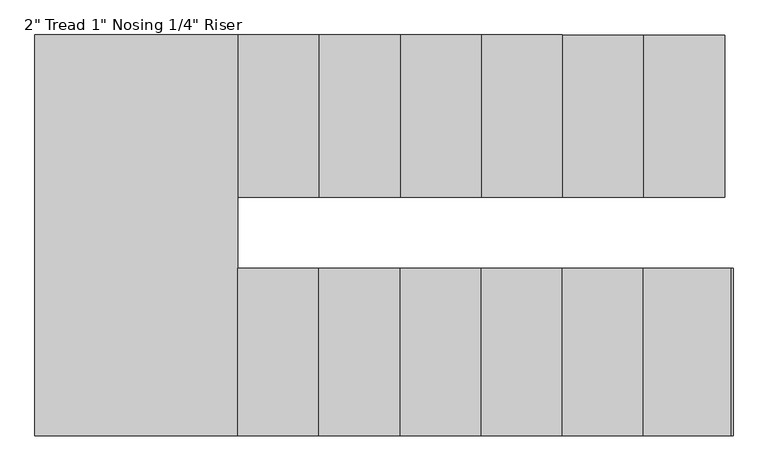
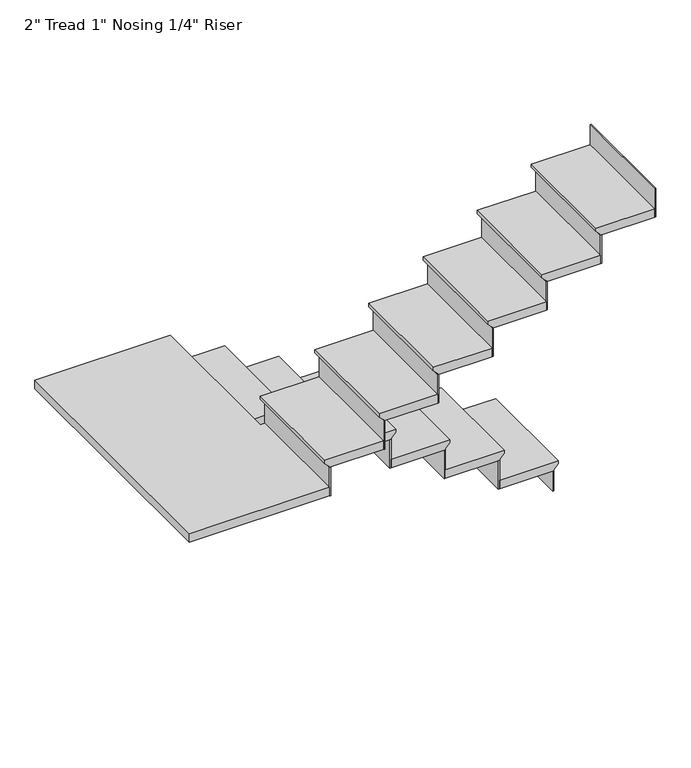
"""IFC4 building model written with IfcOpenShell, lengths in millimetres: stair flight geometry."""

from ifc_helpers import new_model, si_unit, origin, place, context, project, spatial, faceted_brep, source, transform, mapped, element, save


def stair_flight_b71cab51(model_context):
    return source(origin(), model_context, "Body", "Brep", [
        faceted_brep([(-2968.8120155, -2170.0065691, 3350.6833333), (-2968.8120155, -2170.0065691, 3369.7333333), (-2968.8120155, -2779.6065691, 3369.7333333), (-2968.8120155, -2779.6065691, 3350.6833333), (-2994.2120155, -2170.0065691, 3325.2833333), (-2994.2120155, -2779.6065691, 3325.2833333), (-3299.0120155, -2170.0065691, 3369.7333333), (-3299.0120155, -2779.6065691, 3369.7333333), (-2994.2120155, -2779.6065691, 3318.9333333), (-3299.0120155, -2779.6065691, 3318.9333333), (-3299.0120155, -2170.0065691, 3318.9333333), (-2994.2120155, -2170.0065691, 3318.9333333)], [[[0, 1, 2, 3]], [[4, 0, 3, 5]], [[2, 1, 6, 7]], [[8, 9, 10, 11]], [[2, 7, 9, 8, 5, 3]], [[8, 11, 4, 5]], [[6, 1, 0, 4, 11, 10]], [[7, 6, 10, 9]]]),
        faceted_brep([(-2994.2120155, -2170.0065691, 3318.9333333), (-2994.2120155, -2170.0065691, 3200.4), (-3000.5620155, -2170.0065691, 3200.4), (-3000.5620155, -2170.0065691, 3318.9333333), (-2994.2120155, -2779.6065691, 3318.9333333), (-3000.5620155, -2779.6065691, 3318.9333333), (-3000.5620155, -2779.6065691, 3200.4), (-2994.2120155, -2779.6065691, 3200.4)], [[[0, 1, 2, 3]], [[4, 5, 6, 7]], [[1, 0, 4, 7]], [[2, 1, 7, 6]], [[3, 2, 6, 5]], [[0, 3, 5, 4]]]),
        faceted_brep([(-3299.0120155, -2170.0065691, 3488.2666667), (-3299.0120155, -2170.0065691, 3318.9333333), (-3305.3620155, -2170.0065691, 3318.9333333), (-3305.3620155, -2170.0065691, 3488.2666667), (-3299.0120155, -2779.6065691, 3488.2666667), (-3305.3620155, -2779.6065691, 3488.2666667), (-3305.3620155, -2779.6065691, 3318.9333333), (-3299.0120155, -2779.6065691, 3318.9333333)], [[[0, 1, 2, 3]], [[4, 5, 6, 7]], [[1, 0, 4, 7]], [[2, 1, 7, 6]], [[3, 2, 6, 5]], [[0, 3, 5, 4]]]),
        faceted_brep([(-3273.6120155, -2779.6065691, 3539.0666667), (-3273.6120155, -2170.0065691, 3539.0666667), (-3603.8120155, -2170.0065691, 3539.0666667), (-3603.8120155, -2779.6065691, 3539.0666667), (-3299.0120155, -2779.6065691, 3488.2666667), (-3603.8120155, -2779.6065691, 3488.2666667), (-3603.8120155, -2170.0065691, 3488.2666667), (-3299.0120155, -2170.0065691, 3488.2666667), (-3299.0120155, -2779.6065691, 3494.6166667), (-3273.6120155, -2779.6065691, 3520.0166667), (-3299.0120155, -2170.0065691, 3494.6166667), (-3273.6120155, -2170.0065691, 3520.0166667)], [[[0, 1, 2, 3]], [[4, 5, 6, 7]], [[0, 3, 5, 4, 8, 9]], [[4, 7, 10, 8]], [[2, 1, 11, 10, 7, 6]], [[3, 2, 6, 5]], [[11, 1, 0, 9]], [[10, 11, 9, 8]]]),
        faceted_brep([(-3603.8120155, -2170.0065691, 3657.6), (-3603.8120155, -2170.0065691, 3488.2666667), (-3610.1620155, -2170.0065691, 3488.2666667), (-3610.1620155, -2170.0065691, 3657.6), (-3603.8120155, -2779.6065691, 3657.6), (-3610.1620155, -2779.6065691, 3657.6), (-3610.1620155, -2779.6065691, 3488.2666667), (-3603.8120155, -2779.6065691, 3488.2666667)], [[[0, 1, 2, 3]], [[4, 5, 6, 7]], [[1, 0, 4, 7]], [[2, 1, 7, 6]], [[3, 2, 6, 5]], [[0, 3, 5, 4]]]),
        faceted_brep([(-3578.4120155, -2779.6065691, 3708.4), (-3578.4120155, -2170.0065691, 3708.4), (-3908.6120155, -2170.0065691, 3708.4), (-3908.6120155, -2779.6065691, 3708.4), (-3603.8120155, -2779.6065691, 3657.6), (-3908.6120155, -2779.6065691, 3657.6), (-3908.6120155, -2170.0065691, 3657.6), (-3603.8120155, -2170.0065691, 3657.6), (-3603.8120155, -2779.6065691, 3663.95), (-3578.4120155, -2779.6065691, 3689.35), (-3603.8120155, -2170.0065691, 3663.95), (-3578.4120155, -2170.0065691, 3689.35)], [[[0, 1, 2, 3]], [[4, 5, 6, 7]], [[0, 3, 5, 4, 8, 9]], [[4, 7, 10, 8]], [[2, 1, 11, 10, 7, 6]], [[3, 2, 6, 5]], [[11, 1, 0, 9]], [[10, 11, 9, 8]]]),
        faceted_brep([(-3908.6120155, -2170.0065691, 3826.9333333), (-3908.6120155, -2170.0065691, 3657.6), (-3914.9620155, -2170.0065691, 3657.6), (-3914.9620155, -2170.0065691, 3826.9333333), (-3908.6120155, -2779.6065691, 3826.9333333), (-3914.9620155, -2779.6065691, 3826.9333333), (-3914.9620155, -2779.6065691, 3657.6), (-3908.6120155, -2779.6065691, 3657.6)], [[[0, 1, 2, 3]], [[4, 5, 6, 7]], [[1, 0, 4, 7]], [[2, 1, 7, 6]], [[3, 2, 6, 5]], [[0, 3, 5, 4]]]),
        faceted_brep([(-3883.2120155, -2779.6065691, 3877.7333333), (-3883.2120155, -2170.0065691, 3877.7333333), (-4213.4120155, -2170.0065691, 3877.7333333), (-4213.4120155, -2779.6065691, 3877.7333333), (-3908.6120155, -2779.6065691, 3826.9333333), (-4213.4120155, -2779.6065691, 3826.9333333), (-4213.4120155, -2170.0065691, 3826.9333333), (-3908.6120155, -2170.0065691, 3826.9333333), (-3908.6120155, -2779.6065691, 3833.2833333), (-3883.2120155, -2779.6065691, 3858.6833333), (-3908.6120155, -2170.0065691, 3833.2833333), (-3883.2120155, -2170.0065691, 3858.6833333)], [[[0, 1, 2, 3]], [[4, 5, 6, 7]], [[0, 3, 5, 4, 8, 9]], [[4, 7, 10, 8]], [[2, 1, 11, 10, 7, 6]], [[3, 2, 6, 5]], [[11, 1, 0, 9]], [[10, 11, 9, 8]]]),
        faceted_brep([(-4213.4120155, -2170.0065691, 3996.2666667), (-4213.4120155, -2170.0065691, 3826.9333333), (-4219.7620155, -2170.0065691, 3826.9333333), (-4219.7620155, -2170.0065691, 3996.2666667), (-4213.4120155, -2779.6065691, 3996.2666667), (-4219.7620155, -2779.6065691, 3996.2666667), (-4219.7620155, -2779.6065691, 3826.9333333), (-4213.4120155, -2779.6065691, 3826.9333333)], [[[0, 1, 2, 3]], [[4, 5, 6, 7]], [[1, 0, 4, 7]], [[2, 1, 7, 6]], [[3, 2, 6, 5]], [[0, 3, 5, 4]]]),
        faceted_brep([(-4188.0120155, -2779.6065691, 4047.0666667), (-4188.0120155, -2170.0065691, 4047.0666667), (-4518.2120155, -2170.0065691, 4047.0666667), (-4518.2120155, -2779.6065691, 4047.0666667), (-4213.4120155, -2779.6065691, 3996.2666667), (-4518.2120155, -2779.6065691, 3996.2666667), (-4518.2120155, -2170.0065691, 3996.2666667), (-4213.4120155, -2170.0065691, 3996.2666667), (-4213.4120155, -2779.6065691, 4002.6166667), (-4188.0120155, -2779.6065691, 4028.0166667), (-4213.4120155, -2170.0065691, 4002.6166667), (-4188.0120155, -2170.0065691, 4028.0166667)], [[[0, 1, 2, 3]], [[4, 5, 6, 7]], [[0, 3, 5, 4, 8, 9]], [[4, 7, 10, 8]], [[2, 1, 11, 10, 7, 6]], [[3, 2, 6, 5]], [[11, 1, 0, 9]], [[10, 11, 9, 8]]]),
        faceted_brep([(-4518.2120155, -2170.0065691, 4165.6), (-4518.2120155, -2170.0065691, 3996.2666667), (-4524.5620155, -2170.0065691, 3996.2666667), (-4524.5620155, -2170.0065691, 4165.6), (-4518.2120155, -2779.6065691, 4165.6), (-4524.5620155, -2779.6065691, 4165.6), (-4524.5620155, -2779.6065691, 3996.2666667), (-4518.2120155, -2779.6065691, 3996.2666667)], [[[0, 1, 2, 3]], [[4, 5, 6, 7]], [[1, 0, 4, 7]], [[2, 1, 7, 6]], [[3, 2, 6, 5]], [[0, 3, 5, 4]]]),
        faceted_brep([(-4492.8120155, -2779.6065691, 4216.4), (-4492.8120155, -2170.0065691, 4216.4), (-4823.0120155, -2170.0065691, 4216.4), (-4823.0120155, -2779.6065691, 4216.4), (-4518.2120155, -2779.6065691, 4165.6), (-4823.0120155, -2779.6065691, 4165.6), (-4823.0120155, -2170.0065691, 4165.6), (-4518.2120155, -2170.0065691, 4165.6), (-4518.2120155, -2779.6065691, 4171.95), (-4492.8120155, -2779.6065691, 4197.35), (-4518.2120155, -2170.0065691, 4171.95), (-4492.8120155, -2170.0065691, 4197.35)], [[[0, 1, 2, 3]], [[4, 5, 6, 7]], [[0, 3, 5, 4, 8, 9]], [[4, 7, 10, 8]], [[2, 1, 11, 10, 7, 6]], [[3, 2, 6, 5]], [[11, 1, 0, 9]], [[10, 11, 9, 8]]]),
        faceted_brep([(-4823.0120155, -2170.0065691, 4334.9333333), (-4823.0120155, -2170.0065691, 4165.6), (-4829.3620155, -2170.0065691, 4165.6), (-4829.3620155, -2170.0065691, 4334.9333333), (-4823.0120155, -2779.6065691, 4334.9333333), (-4829.3620155, -2779.6065691, 4334.9333333), (-4829.3620155, -2779.6065691, 4165.6), (-4823.0120155, -2779.6065691, 4165.6)], [[[0, 1, 2, 3]], [[4, 5, 6, 7]], [[1, 0, 4, 7]], [[2, 1, 7, 6]], [[3, 2, 6, 5]], [[0, 3, 5, 4]]]),
        faceted_brep([(-4772.2120155, -3046.3065691, 4385.7333333), (-4797.6120155, -3046.3065691, 4385.7333333), (-4797.6120155, -2170.0065691, 4385.7333333), (-5559.6120155, -2170.0065691, 4385.7333333), (-5559.6120155, -3674.9565691, 4385.7333333), (-4772.2120155, -3674.9565691, 4385.7333333), (-4797.6120155, -3046.3065691, 4334.9333333), (-4772.2120155, -3046.3065691, 4334.9333333), (-4772.2120155, -3674.9565691, 4334.9333333), (-5559.6120155, -3674.9565691, 4334.9333333), (-5559.6120155, -2170.0065691, 4334.9333333), (-4823.0120155, -2170.0065691, 4334.9333333), (-4823.0120155, -2779.6065691, 4334.9333333), (-4797.6120155, -2779.6065691, 4334.9333333), (-4797.6120155, -2779.6065691, 4366.6833333), (-4797.6120155, -2170.0065691, 4366.6833333), (-4823.0120155, -2779.6065691, 4341.2833333), (-4823.0120155, -2170.0065691, 4341.2833333)], [[[0, 1, 2, 3, 4, 5]], [[6, 7, 8, 9, 10, 11, 12, 13]], [[1, 0, 7, 6]], [[2, 1, 6, 13, 14, 15]], [[13, 12, 16, 14]], [[12, 11, 17, 16]], [[3, 2, 15, 17, 11, 10]], [[4, 3, 10, 9]], [[5, 4, 9, 8]], [[0, 5, 8, 7]], [[17, 15, 14, 16]]]),
        faceted_brep([(-4772.2120155, -3674.9565691, 4504.2666667), (-4772.2120155, -3674.9565691, 4334.9333333), (-4765.8620155, -3674.9565691, 4334.9333333), (-4765.8620155, -3674.9565691, 4504.2666667), (-4772.2120155, -3046.3065691, 4504.2666667), (-4765.8620155, -3046.3065691, 4504.2666667), (-4765.8620155, -3046.3065691, 4334.9333333), (-4772.2120155, -3046.3065691, 4334.9333333)], [[[0, 1, 2, 3]], [[4, 5, 6, 7]], [[1, 0, 4, 7]], [[2, 1, 7, 6]], [[3, 2, 6, 5]], [[0, 3, 5, 4]]]),
        faceted_brep([(-4797.6120155, -3046.3065691, 4555.0666667), (-4797.6120155, -3674.9565691, 4555.0666667), (-4467.4120155, -3674.9565691, 4555.0666667), (-4467.4120155, -3046.3065691, 4555.0666667), (-4772.2120155, -3046.3065691, 4504.2666667), (-4467.4120155, -3046.3065691, 4504.2666667), (-4467.4120155, -3674.9565691, 4504.2666667), (-4772.2120155, -3674.9565691, 4504.2666667), (-4772.2120155, -3046.3065691, 4510.6166667), (-4797.6120155, -3046.3065691, 4536.0166667), (-4772.2120155, -3674.9565691, 4510.6166667), (-4797.6120155, -3674.9565691, 4536.0166667)], [[[0, 1, 2, 3]], [[4, 5, 6, 7]], [[0, 3, 5, 4, 8, 9]], [[4, 7, 10, 8]], [[2, 1, 11, 10, 7, 6]], [[3, 2, 6, 5]], [[11, 1, 0, 9]], [[10, 11, 9, 8]]]),
        faceted_brep([(-4467.4120155, -3674.9565691, 4673.6), (-4467.4120155, -3674.9565691, 4504.2666667), (-4461.0620155, -3674.9565691, 4504.2666667), (-4461.0620155, -3674.9565691, 4673.6), (-4467.4120155, -3046.3065691, 4673.6), (-4461.0620155, -3046.3065691, 4673.6), (-4461.0620155, -3046.3065691, 4504.2666667), (-4467.4120155, -3046.3065691, 4504.2666667)], [[[0, 1, 2, 3]], [[4, 5, 6, 7]], [[1, 0, 4, 7]], [[2, 1, 7, 6]], [[3, 2, 6, 5]], [[0, 3, 5, 4]]]),
        faceted_brep([(-4492.8120155, -3046.3065691, 4724.4), (-4492.8120155, -3674.9565691, 4724.4), (-4162.6120155, -3674.9565691, 4724.4), (-4162.6120155, -3046.3065691, 4724.4), (-4467.4120155, -3046.3065691, 4673.6), (-4162.6120155, -3046.3065691, 4673.6), (-4162.6120155, -3674.9565691, 4673.6), (-4467.4120155, -3674.9565691, 4673.6), (-4467.4120155, -3046.3065691, 4679.95), (-4492.8120155, -3046.3065691, 4705.35), (-4467.4120155, -3674.9565691, 4679.95), (-4492.8120155, -3674.9565691, 4705.35)], [[[0, 1, 2, 3]], [[4, 5, 6, 7]], [[0, 3, 5, 4, 8, 9]], [[4, 7, 10, 8]], [[2, 1, 11, 10, 7, 6]], [[3, 2, 6, 5]], [[11, 1, 0, 9]], [[10, 11, 9, 8]]]),
        faceted_brep([(-4162.6120155, -3674.9565691, 4842.9333333), (-4162.6120155, -3674.9565691, 4673.6), (-4156.2620155, -3674.9565691, 4673.6), (-4156.2620155, -3674.9565691, 4842.9333333), (-4162.6120155, -3046.3065691, 4842.9333333), (-4156.2620155, -3046.3065691, 4842.9333333), (-4156.2620155, -3046.3065691, 4673.6), (-4162.6120155, -3046.3065691, 4673.6)], [[[0, 1, 2, 3]], [[4, 5, 6, 7]], [[1, 0, 4, 7]], [[2, 1, 7, 6]], [[3, 2, 6, 5]], [[0, 3, 5, 4]]]),
        faceted_brep([(-4188.0120155, -3046.3065691, 4893.7333333), (-4188.0120155, -3674.9565691, 4893.7333333), (-3857.8120155, -3674.9565691, 4893.7333333), (-3857.8120155, -3046.3065691, 4893.7333333), (-4162.6120155, -3046.3065691, 4842.9333333), (-3857.8120155, -3046.3065691, 4842.9333333), (-3857.8120155, -3674.9565691, 4842.9333333), (-4162.6120155, -3674.9565691, 4842.9333333), (-4162.6120155, -3046.3065691, 4849.2833333), (-4188.0120155, -3046.3065691, 4874.6833333), (-4162.6120155, -3674.9565691, 4849.2833333), (-4188.0120155, -3674.9565691, 4874.6833333)], [[[0, 1, 2, 3]], [[4, 5, 6, 7]], [[0, 3, 5, 4, 8, 9]], [[4, 7, 10, 8]], [[2, 1, 11, 10, 7, 6]], [[3, 2, 6, 5]], [[11, 1, 0, 9]], [[10, 11, 9, 8]]]),
        faceted_brep([(-3857.8120155, -3674.9565691, 5012.2666667), (-3857.8120155, -3674.9565691, 4842.9333333), (-3851.4620155, -3674.9565691, 4842.9333333), (-3851.4620155, -3674.9565691, 5012.2666667), (-3857.8120155, -3046.3065691, 5012.2666667), (-3851.4620155, -3046.3065691, 5012.2666667), (-3851.4620155, -3046.3065691, 4842.9333333), (-3857.8120155, -3046.3065691, 4842.9333333)], [[[0, 1, 2, 3]], [[4, 5, 6, 7]], [[1, 0, 4, 7]], [[2, 1, 7, 6]], [[3, 2, 6, 5]], [[0, 3, 5, 4]]]),
        faceted_brep([(-3883.2120155, -3046.3065691, 5063.0666667), (-3883.2120155, -3674.9565691, 5063.0666667), (-3553.0120155, -3674.9565691, 5063.0666667), (-3553.0120155, -3046.3065691, 5063.0666667), (-3857.8120155, -3046.3065691, 5012.2666667), (-3553.0120155, -3046.3065691, 5012.2666667), (-3553.0120155, -3674.9565691, 5012.2666667), (-3857.8120155, -3674.9565691, 5012.2666667), (-3857.8120155, -3046.3065691, 5018.6166667), (-3883.2120155, -3046.3065691, 5044.0166667), (-3857.8120155, -3674.9565691, 5018.6166667), (-3883.2120155, -3674.9565691, 5044.0166667)], [[[0, 1, 2, 3]], [[4, 5, 6, 7]], [[0, 3, 5, 4, 8, 9]], [[4, 7, 10, 8]], [[2, 1, 11, 10, 7, 6]], [[3, 2, 6, 5]], [[11, 1, 0, 9]], [[10, 11, 9, 8]]]),
        faceted_brep([(-3553.0120155, -3674.9565691, 5181.6), (-3553.0120155, -3674.9565691, 5012.2666667), (-3546.6620155, -3674.9565691, 5012.2666667), (-3546.6620155, -3674.9565691, 5181.6), (-3553.0120155, -3046.3065691, 5181.6), (-3546.6620155, -3046.3065691, 5181.6), (-3546.6620155, -3046.3065691, 5012.2666667), (-3553.0120155, -3046.3065691, 5012.2666667)], [[[0, 1, 2, 3]], [[4, 5, 6, 7]], [[1, 0, 4, 7]], [[2, 1, 7, 6]], [[3, 2, 6, 5]], [[0, 3, 5, 4]]]),
        faceted_brep([(-3578.4120155, -3046.3065691, 5232.4), (-3578.4120155, -3674.9565691, 5232.4), (-3248.2120155, -3674.9565691, 5232.4), (-3248.2120155, -3046.3065691, 5232.4), (-3553.0120155, -3046.3065691, 5181.6), (-3248.2120155, -3046.3065691, 5181.6), (-3248.2120155, -3674.9565691, 5181.6), (-3553.0120155, -3674.9565691, 5181.6), (-3553.0120155, -3046.3065691, 5187.95), (-3578.4120155, -3046.3065691, 5213.35), (-3553.0120155, -3674.9565691, 5187.95), (-3578.4120155, -3674.9565691, 5213.35)], [[[0, 1, 2, 3]], [[4, 5, 6, 7]], [[0, 3, 5, 4, 8, 9]], [[4, 7, 10, 8]], [[2, 1, 11, 10, 7, 6]], [[3, 2, 6, 5]], [[11, 1, 0, 9]], [[10, 11, 9, 8]]]),
        faceted_brep([(-3248.2120155, -3674.9565691, 5350.9333333), (-3248.2120155, -3674.9565691, 5181.6), (-3241.8620155, -3674.9565691, 5181.6), (-3241.8620155, -3674.9565691, 5350.9333333), (-3248.2120155, -3046.3065691, 5350.9333333), (-3241.8620155, -3046.3065691, 5350.9333333), (-3241.8620155, -3046.3065691, 5181.6), (-3248.2120155, -3046.3065691, 5181.6)], [[[0, 1, 2, 3]], [[4, 5, 6, 7]], [[1, 0, 4, 7]], [[2, 1, 7, 6]], [[3, 2, 6, 5]], [[0, 3, 5, 4]]]),
        faceted_brep([(-2943.4120155, -3674.9565691, 5520.2666667), (-2943.4120155, -3674.9565691, 5350.9333333), (-2937.0620155, -3674.9565691, 5350.9333333), (-2937.0620155, -3674.9565691, 5520.2666667), (-2943.4120155, -3046.3065691, 5520.2666667), (-2937.0620155, -3046.3065691, 5520.2666667), (-2937.0620155, -3046.3065691, 5350.9333333), (-2943.4120155, -3046.3065691, 5350.9333333)], [[[0, 1, 2, 3]], [[4, 5, 6, 7]], [[1, 0, 4, 7]], [[2, 1, 7, 6]], [[3, 2, 6, 5]], [[0, 3, 5, 4]]]),
        faceted_brep([(-3273.6120155, -3046.3065691, 5401.7333333), (-3273.6120155, -3674.9565691, 5401.7333333), (-2943.4120155, -3674.9565691, 5401.7333333), (-2943.4120155, -3046.3065691, 5401.7333333), (-3248.2120155, -3046.3065691, 5350.9333333), (-2943.4120155, -3046.3065691, 5350.9333333), (-2943.4120155, -3674.9565691, 5350.9333333), (-3248.2120155, -3674.9565691, 5350.9333333), (-3248.2120155, -3046.3065691, 5357.2833333), (-3273.6120155, -3046.3065691, 5382.6833333), (-3248.2120155, -3674.9565691, 5357.2833333), (-3273.6120155, -3674.9565691, 5382.6833333)], [[[0, 1, 2, 3]], [[4, 5, 6, 7]], [[0, 3, 5, 4, 8, 9]], [[4, 7, 10, 8]], [[2, 1, 11, 10, 7, 6]], [[3, 2, 6, 5]], [[11, 1, 0, 9]], [[10, 11, 9, 8]]]),
    ])


if __name__ == "__main__":
    model = new_model("IFC4")
    model_context = context("Model", 3, world=origin())
    ifc_project = project(units=[si_unit("LENGTHUNIT", "METRE", prefix="MILLI")], contexts=[model_context])
    site = spatial("IfcSite", under=ifc_project)
    building = spatial("IfcBuilding", under=site)
    placement = place(None, origin())
    stair_flight_shape = stair_flight_b71cab51(model_context)
    element("IfcStairFlight", 1, ObjectType="2\" Tread 1\" Nosing 1/4\" Riser", at=placement, inside=building, context=model_context, shape_type="MappedRepresentation", body=[
        mapped(stair_flight_shape, transform((0.0, 0.0, 0.0), x_axis=(1.0, 0.0, 0.0), y_axis=(0.0, 1.0, 0.0), z_axis=(0.0, 0.0, 1.0))),
    ])
    save(model, "model.ifc")
